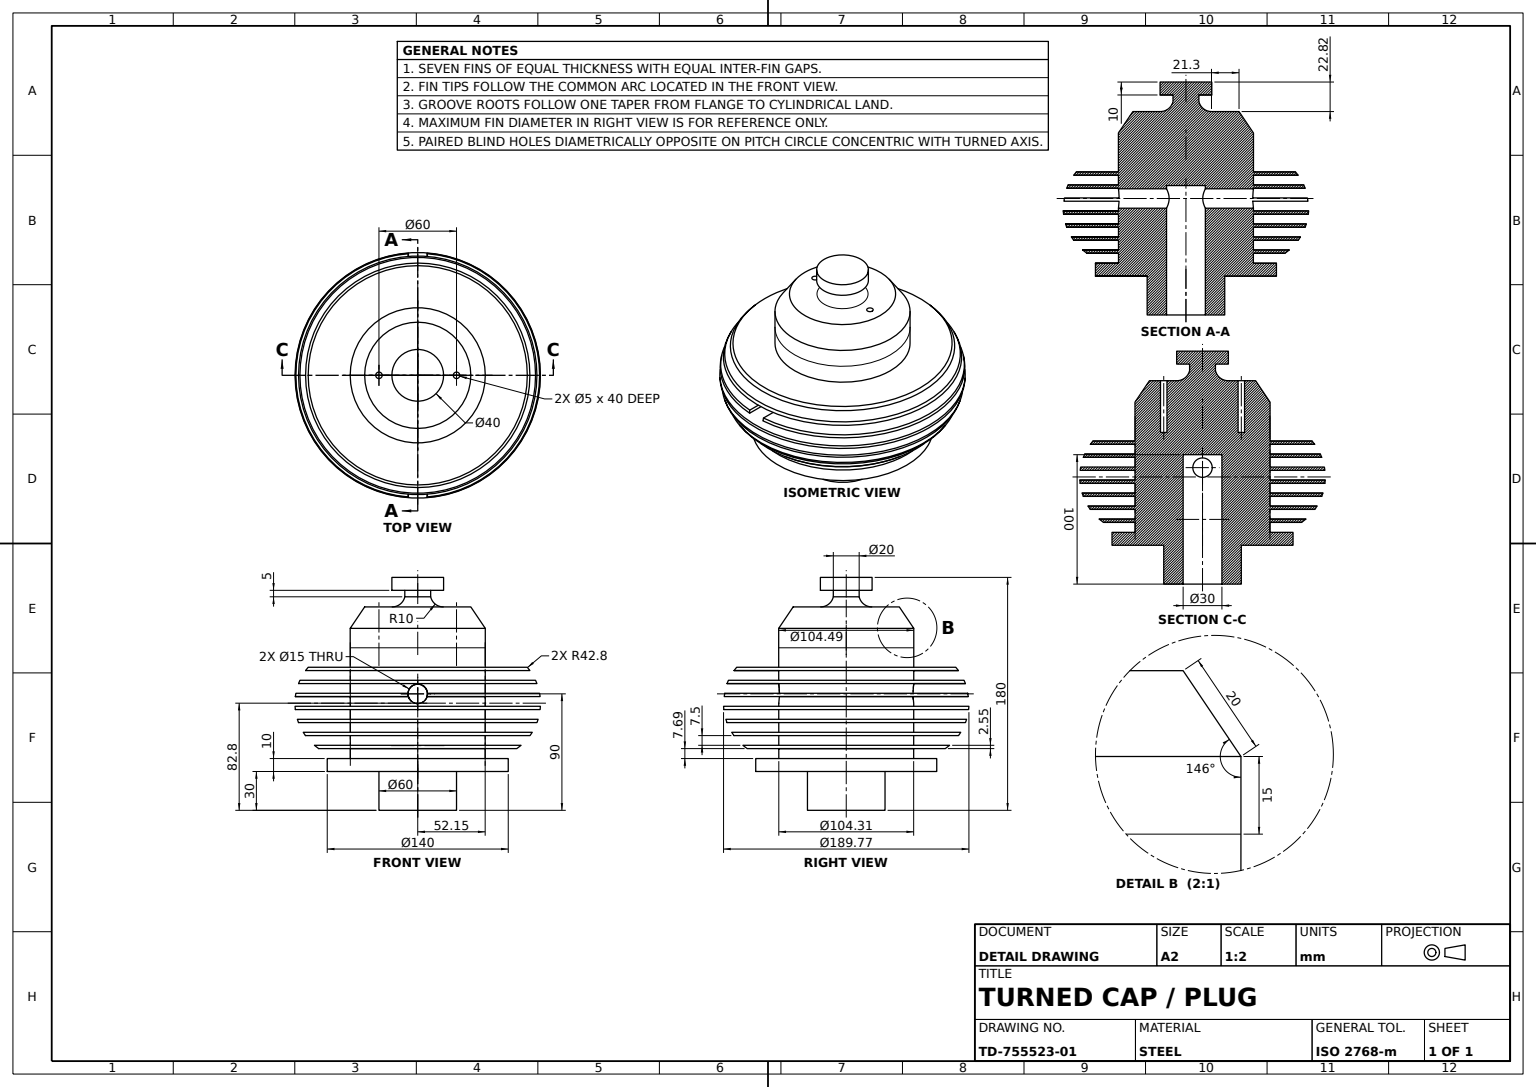
SolidWorks part; units mm, degrees
material "Plain Carbon Steel"
ref_plane "Front Plane" through (0, 0, 0) normal (0, 0, 1) x (1, 0, 0)
ref_plane "Top Plane" through (0, 0, 0) normal (0, 1, 0) x (1, 0, 0)
ref_plane "Right Plane" through (0, 0, 0) normal (1, 0, 0) x (0, 0, -1)
sketch "Turned Body Profile" plane through (0, 0, 0) normal (0, 0, 1) x (1, 0, 0)
  line L0 (-64.3435, 0) -> (66.4275, 0) construction
  line L1 (0, 35.4801) -> (0, -173.9212) construction
  line L2 (0, 26.5584) -> (20, 26.5584)
  line L3 (20, 26.5584) -> (20, 16.5584)
  line L4 (20, 16.5584) -> (10, 16.5584)
  line L5 (10, 16.5584) -> (10, 11.5584)
  line L6 (19.7593, 3.739) -> (41.0593, 3.739)
  line L7 (41.0593, 3.739) -> (52.2432, -12.8417)
  line L8 (52.2432, -12.8417) -> (52.2432, -27.8417)
  line L12 (30, -123.4416) -> (30, -153.4416)
  line L13 (30, -153.4416) -> (0, -153.4416)
  line L14 (0, 26.5584) -> (0, -153.4416)
  line L15 (52.2432, -27.8417) -> (52.238, -32.8417)
  line L16 (52.238, -32.8417) -> (72.229, -32.8417)
  line L17 (76.4306, -35.3927) -> (52.2353, -35.3927)
  line L19 (52.238, -32.8417) -> (52.2353, -35.3927)
  line L20 (86.7503, -45.4437) -> (52.2249, -45.4437)
  line L21 (52.2275, -42.8927) -> (84.7398, -42.8927)
  line L22 (52.162, -105.7495) -> (52.154, -113.4416)
  line L23 (92.1841, -55.4947) -> (52.2144, -55.4947)
  line L24 (52.217, -52.9437) -> (91.1235, -52.9437)
  line L25 (52.1725, -95.6985) -> (52.1647, -103.1985)
  line L26 (94.6495, -65.5456) -> (52.2039, -65.5456)
  line L27 (52.2066, -62.9946) -> (94.2653, -62.9946)
  line L28 (52.183, -85.6476) -> (52.1752, -93.1476)
  line L29 (94.6662, -75.5966) -> (52.1934, -75.5966)
  line L30 (52.1961, -73.0456) -> (94.8864, -73.0456)
  line L31 (52.1934, -75.5966) -> (52.1856, -83.0966)
  line L32 (92.2372, -85.6476) -> (52.183, -85.6476)
  line L33 (52.1856, -83.0966) -> (93.1017, -83.0966)
  line L34 (52.2039, -65.5456) -> (52.1961, -73.0456)
  line L35 (86.8526, -95.6985) -> (52.1725, -95.6985)
  line L36 (52.1752, -93.1476) -> (88.559, -93.1476)
  line L37 (52.2144, -55.4947) -> (52.2066, -62.9946)
  line L38 (76.6342, -105.7495) -> (51.8851, -105.7495)
  line L39 (52.1647, -103.1985) -> (79.9369, -103.1985)
  line L40 (52.2249, -45.4437) -> (52.217, -52.9437)
  line L41 (30, -123.4416) -> (70, -123.4416)
  line L42 (70, -123.4416) -> (70, -113.4416)
  line L43 (70, -113.4416) -> (52.154, -113.4416)
  line L48 (52.2353, -35.3927) -> (52.2275, -42.8927)
  line L49 (52.2432, -27.8417) -> (52.238, -32.8417)
  arc A0 (10, 11.5584) -> (19.7593, 3.739) centre (19.7593, 13.739) ccw
  arc A1 (72.229, -32.8417) -> (76.4306, -35.3927) centre (52.154, -70.6416) cw
  arc A2 (93.1017, -83.0966) -> (92.2372, -85.6476) centre (52.154, -70.6416) cw
  arc A3 (94.8864, -73.0456) -> (94.6662, -75.5966) centre (52.154, -70.6416) cw
  arc A4 (94.2653, -62.9946) -> (94.6495, -65.5456) centre (52.154, -70.6416) cw
  arc A5 (91.1235, -52.9437) -> (92.1841, -55.4947) centre (52.154, -70.6416) cw
  arc A6 (84.7398, -42.8927) -> (86.7503, -45.4437) centre (52.154, -70.6416) cw
  arc A7 (79.9369, -103.1985) -> (76.6342, -105.7495) centre (52.154, -70.6416) cw
  arc A8 (88.559, -93.1476) -> (86.8526, -95.6985) centre (52.154, -70.6416) cw
  dimension "D5" = 10
  dimension "D10" = 42.8
  dimension "D18" = 52.154
  dimension "D1" = 20
  dimension "D2" = 10
  dimension "D3" = 10
  dimension "D4" = 5
  dimension "D6" = 21.3
  dimension "D7" = 20
  dimension "D8" = 15
  dimension "D9" = 146
  dimension "D11" = 180
  dimension "D12" = 10
  dimension "D13" = 40
  dimension "D14" = 30
  dimension "D15" = 30
  dimension "D16" = 26.5584
  dimension "D17" = 3.739
  dimension "D19" = 5
  dimension "D21" = 7.5
  dimension "D22" = 42.8
  dimension "D23" = 2.551
  dimension "D24" = 24.749
  dimension "D20" = 8
revolve "Turned Body" add sketch "Turned Body Profile" angle 360 about L1
sketch "Cut Ø30 Sketch" plane through (0, -153.4416, 0) normal (0, -1, 0) x (1, 0, 0)
  circle A0 centre (0, 0) radius 15
  dimension "D1" = 30
extrude "Cut Ø30" cut sketch "Cut Ø30 Sketch" against normal blind 100
sketch "Rectangular Cut Sketch" plane through (0, 3.739, 0) normal (0, 1, 0) x (1, 0, 0)
  line L0 (-133.7046, 0) -> (155.4736, 0) construction
  line L1 (0, 111.7475) -> (0, -115.94) construction
  circle A0 centre (30, 0) radius 2.5
  circle A1 centre (-30, 0) radius 2.5
  dimension "D1" = 5
  dimension "D2" = 5
  dimension "D3" = 30
  dimension "D4" = 30
extrude "Rectangular Cut 40 Deep" cut sketch "Rectangular Cut Sketch" against normal blind 40
sketch "Front Plane Cut Sketch" plane through (0, 0, 0) normal (0, 0, 1) x (1, 0, 0)
  line L0 (0, 26.5584) -> (0, -153.4416) construction
  line L1 (20, 26.5584) -> (-20, 26.5584) construction
  line L2 (-30, -153.4416) -> (30, -153.4416) construction
  circle A0 centre (0, -63.4416) radius 7.5
  dimension "D1" = 15
extrude "Front Plane Cut" cut sketch "Front Plane Cut Sketch" against normal through all both and the other way through all
